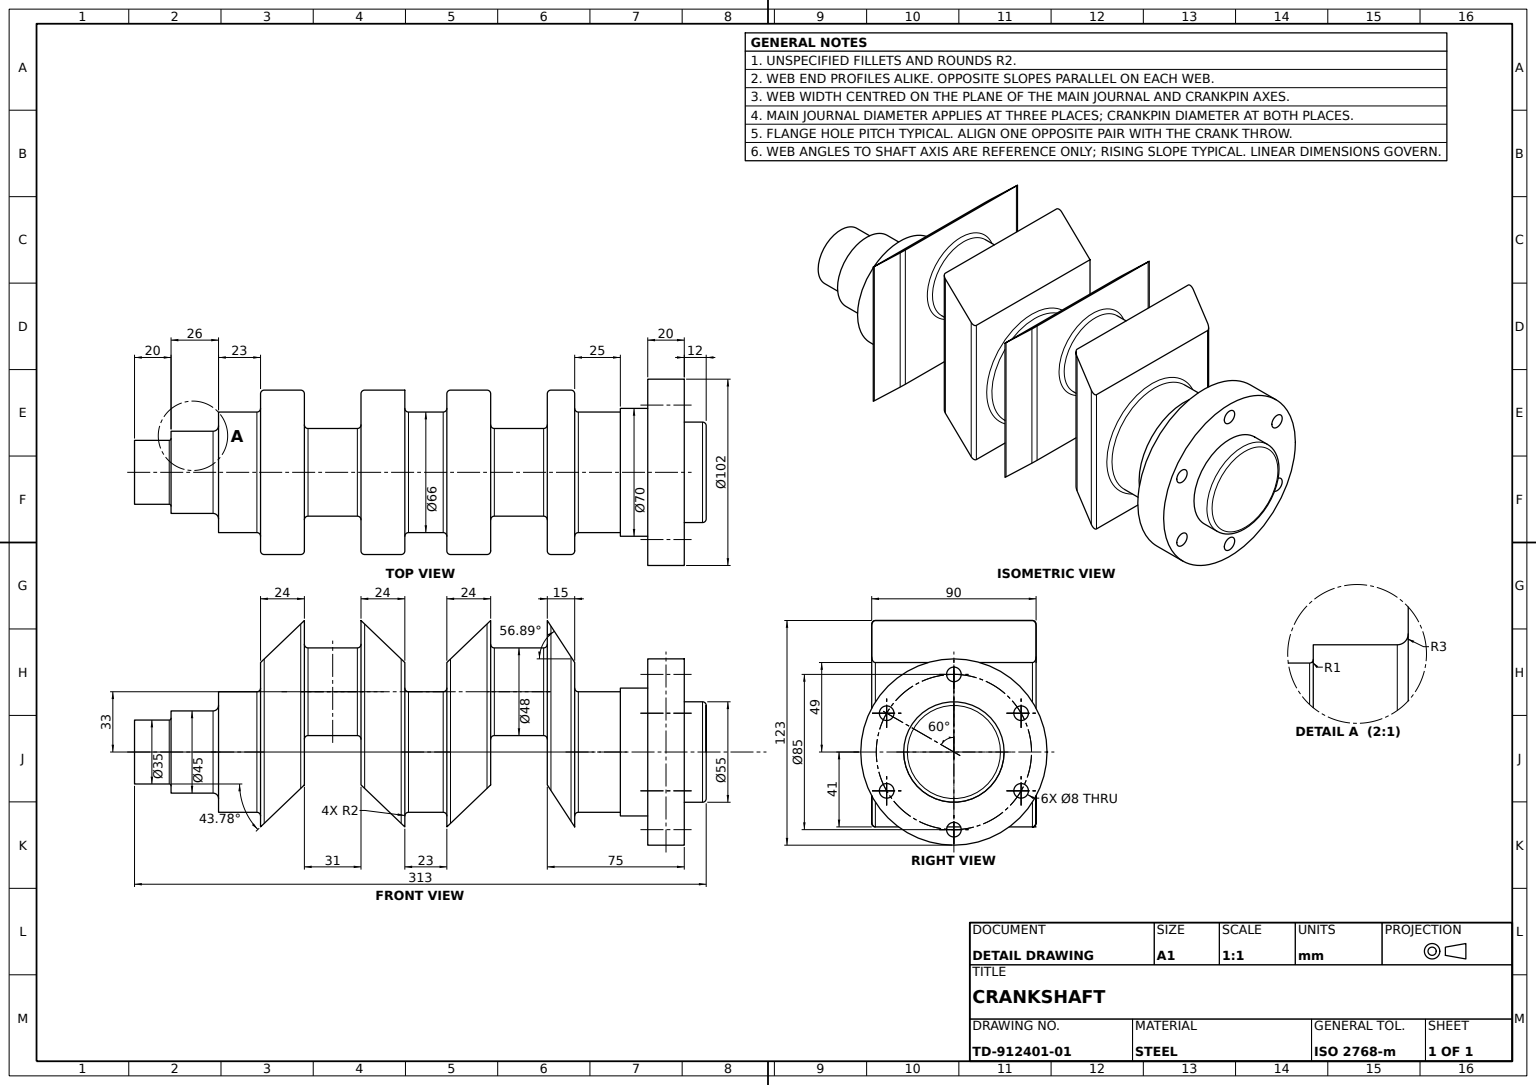
from build123d import *

# Parameters (mm, degrees)
FRONT_JOURNAL_35_SKETCH_R          = 17.5
FRONT_JOURNAL_35_DEPTH             = 20
SHAFT_STEP_45_SKETCH_R             = 22.5
SHAFT_STEP_45_DEPTH                = 26
FRONT_MAIN_JOURNAL_66_SKETCH_R     = 33
FRONT_MAIN_JOURNAL_66_DEPTH        = 23
CRANK_WEB_1_DEPTH                  = 45
CRANKPIN_1_48_SKETCH_R             = 24
CRANKPIN_1_48_DEPTH                = 31
CRANK_WEB_2_DEPTH                  = 45
CENTRE_MAIN_JOURNAL_66_SKETCH_R    = 33
CENTRE_MAIN_JOURNAL_66_DEPTH       = 23
CRANK_WEB_3_DEPTH                  = 45
CRANKPIN_2_SKETCH_R                = 24
CRANKPIN_2_DEPTH                   = 31
CRANK_WEB_4_DEPTH                  = 45
REAR_MAIN_JOURNAL_SKETCH_R         = 33
REAR_MAIN_JOURNAL_DEPTH            = 25
FLANGE_NECK_70_SKETCH_R            = 35
FLANGE_NECK_70_DEPTH               = 15
REAR_FLANGE_102_SKETCH_R           = 51
REAR_FLANGE_102_DEPTH              = 20
FLANGE_SPIGOT_55_SKETCH_R          = 27.5
FLANGE_SPIGOT_55_DEPTH             = 12
FLANGE_BOLT_HOLES_6X_8_PCD85_REACH = 315.665
FLANGE_BOLT_HOLES_SKETCH_R         = 4
FRONT_JOURNAL_FILLET_R1_R          = 1
SHAFT_STEP_FILLET_R3_R             = 3
JOURNAL_AND_CRANKPIN_FILLETS_R2_R  = 2
CRANK_WEB_1_EDGE_FILLET_R2_R       = 2
CRANK_WEBS_2_4_EDGE_FILLETS_R2_R   = 2


with BuildPart() as part:
    # Front Journal Ø35 Sketch → Front Journal Ø35 (new body)
    with BuildSketch(Plane.XY):
        Circle(FRONT_JOURNAL_35_SKETCH_R)
    extrude(amount=-FRONT_JOURNAL_35_DEPTH)

    # Shaft Step Ø45 Sketch → Shaft Step Ø45 (add)
    with BuildSketch(Plane(origin=(0, 0, -20), x_dir=(-1, 0, 0), z_dir=(0, 0, -1))):
        with Locations(Location((0, 0, 0), (0, 0, 180))):
            Circle(SHAFT_STEP_45_SKETCH_R)
    extrude(amount=SHAFT_STEP_45_DEPTH)

    # Front Main Journal Ø66 Sketch → Front Main Journal Ø66 (add)
    with BuildSketch(Plane(origin=(0, 0, -46), x_dir=(-1, 0, 0), z_dir=(0, 0, -1))):
        Circle(FRONT_MAIN_JOURNAL_66_SKETCH_R)
    extrude(amount=FRONT_MAIN_JOURNAL_66_DEPTH)

    # Crank Web 1 Profile → Crank Web 1 (add, symmetric)
    with BuildSketch(Plane(origin=(0, 0, 0), x_dir=(0, 0, -1), z_dir=(1, 0, 0))):
        Polygon((69, 0), (69, 49), (93, 72), (93, -18), (69, -41), align=None)
    extrude(amount=CRANK_WEB_1_DEPTH, both=True)

    # Crankpin 1 Ø48 Sketch → Crankpin 1 Ø48 (add)
    with BuildSketch(Plane(origin=(0, 0, -93), x_dir=(-1, 0, 0), z_dir=(0, 0, -1))):
        with Locations(Location((0, 33, 0), (0, 0, 90))):
            Circle(CRANKPIN_1_48_SKETCH_R)
    extrude(amount=CRANKPIN_1_48_DEPTH)

    # Crank Web 2 Profile → Crank Web 2 (add, symmetric)
    with BuildSketch(Plane(origin=(0, 0, 0), x_dir=(0, 0, -1), z_dir=(1, 0, 0))):
        Polygon((124, 72), (124, -18), (148, -41), (148, 49), align=None)
    extrude(amount=CRANK_WEB_2_DEPTH, both=True)

    # Centre Main Journal Ø66 Sketch → Centre Main Journal Ø66 (add)
    with BuildSketch(Plane(origin=(0, 0, -148), x_dir=(-1, 0, 0), z_dir=(0, 0, -1))):
        Circle(CENTRE_MAIN_JOURNAL_66_SKETCH_R)
    extrude(amount=CENTRE_MAIN_JOURNAL_66_DEPTH)

    # Crank Web 3 Profile → Crank Web 3 (add, symmetric)
    with BuildSketch(Plane(origin=(0, 0, 0), x_dir=(0, 0, -1), z_dir=(1, 0, 0))):
        Polygon((171, 0), (171, 49), (195, 72), (195, -18), (171, -41), align=None)
    extrude(amount=CRANK_WEB_3_DEPTH, both=True)

    # Crankpin 2 Sketch → Crankpin 2 (add)
    with BuildSketch(Plane(origin=(0, 0, -195), x_dir=(-1, 0, 0), z_dir=(0, 0, -1))):
        with Locations(Location((0, 33, 0), (0, 0, 90))):
            Circle(CRANKPIN_2_SKETCH_R)
    extrude(amount=CRANKPIN_2_DEPTH)

    # Crank Web 4 Profile → Crank Web 4 (add, symmetric)
    with BuildSketch(Plane(origin=(0, 0, 0), x_dir=(0, 0, -1), z_dir=(1, 0, 0))):
        Polygon((226, 57), (226, 72), (241, 49), (241, -41), (226, -18), align=None)
    extrude(amount=CRANK_WEB_4_DEPTH, both=True)

    # Rear Main Journal Sketch → Rear Main Journal (add)
    with BuildSketch(Plane(origin=(0, 0, -241), x_dir=(-1, 0, 0), z_dir=(0, 0, -1))):
        Circle(REAR_MAIN_JOURNAL_SKETCH_R)
    extrude(amount=REAR_MAIN_JOURNAL_DEPTH)

    # Flange Neck Ø70 Sketch → Flange Neck Ø70 (add)
    with BuildSketch(Plane(origin=(0, 0, -266), x_dir=(-1, 0, 0), z_dir=(0, 0, -1))):
        Circle(FLANGE_NECK_70_SKETCH_R)
    extrude(amount=FLANGE_NECK_70_DEPTH)

    # Rear Flange Ø102 Sketch → Rear Flange Ø102 (add)
    with BuildSketch(Plane(origin=(0, 0, -281), x_dir=(-1, 0, 0), z_dir=(0, 0, -1))):
        Circle(REAR_FLANGE_102_SKETCH_R)
    extrude(amount=REAR_FLANGE_102_DEPTH)

    # Flange Spigot Ø55 Sketch → Flange Spigot Ø55 (add)
    with BuildSketch(Plane(origin=(0, 0, -301), x_dir=(-1, 0, 0), z_dir=(0, 0, -1))):
        Circle(FLANGE_SPIGOT_55_SKETCH_R)
    extrude(amount=FLANGE_SPIGOT_55_DEPTH)

    # Flange Bolt Holes Sketch → Flange Bolt Holes 6xØ8 PCD85 (cut, up to next)
    with BuildSketch(Plane(origin=(0, 0, -301), x_dir=(-1, 0, 0), z_dir=(0, 0, -1)), mode=Mode.PRIVATE) as flange_bolt_holes_6x_8_pcd85_sk1:
        with Locations((0, 42.5)):
            Circle(FLANGE_BOLT_HOLES_SKETCH_R)
    flange_bolt_holes_6x_8_pcd85_tool1 = extrude(flange_bolt_holes_6x_8_pcd85_sk1.sketch, amount=-FLANGE_BOLT_HOLES_6X_8_PCD85_REACH, mode=Mode.PRIVATE) & part.part
    # Flange Bolt Holes Sketch → Flange Bolt Holes 6xØ8 PCD85 (cut, up to next)
    with BuildSketch(Plane(origin=(0, 0, -301), x_dir=(-1, 0, 0), z_dir=(0, 0, -1)), mode=Mode.PRIVATE) as flange_bolt_holes_6x_8_pcd85_sk2:
        with Locations((36.806079661, 21.25)):
            Circle(FLANGE_BOLT_HOLES_SKETCH_R)
    flange_bolt_holes_6x_8_pcd85_tool2 = extrude(flange_bolt_holes_6x_8_pcd85_sk2.sketch, amount=-FLANGE_BOLT_HOLES_6X_8_PCD85_REACH, mode=Mode.PRIVATE) & part.part
    # Flange Bolt Holes Sketch → Flange Bolt Holes 6xØ8 PCD85 (cut, up to next)
    with BuildSketch(Plane(origin=(0, 0, -301), x_dir=(-1, 0, 0), z_dir=(0, 0, -1)), mode=Mode.PRIVATE) as flange_bolt_holes_6x_8_pcd85_sk3:
        with Locations((36.806079661, -21.25)):
            Circle(FLANGE_BOLT_HOLES_SKETCH_R)
    flange_bolt_holes_6x_8_pcd85_tool3 = extrude(flange_bolt_holes_6x_8_pcd85_sk3.sketch, amount=-FLANGE_BOLT_HOLES_6X_8_PCD85_REACH, mode=Mode.PRIVATE) & part.part
    # Flange Bolt Holes Sketch → Flange Bolt Holes 6xØ8 PCD85 (cut, up to next)
    with BuildSketch(Plane(origin=(0, 0, -301), x_dir=(-1, 0, 0), z_dir=(0, 0, -1)), mode=Mode.PRIVATE) as flange_bolt_holes_6x_8_pcd85_sk4:
        with Locations((0, -42.5)):
            Circle(FLANGE_BOLT_HOLES_SKETCH_R)
    flange_bolt_holes_6x_8_pcd85_tool4 = extrude(flange_bolt_holes_6x_8_pcd85_sk4.sketch, amount=-FLANGE_BOLT_HOLES_6X_8_PCD85_REACH, mode=Mode.PRIVATE) & part.part
    # Flange Bolt Holes Sketch → Flange Bolt Holes 6xØ8 PCD85 (cut, up to next)
    with BuildSketch(Plane(origin=(0, 0, -301), x_dir=(-1, 0, 0), z_dir=(0, 0, -1)), mode=Mode.PRIVATE) as flange_bolt_holes_6x_8_pcd85_sk5:
        with Locations((-36.806079661, -21.25)):
            Circle(FLANGE_BOLT_HOLES_SKETCH_R)
    flange_bolt_holes_6x_8_pcd85_tool5 = extrude(flange_bolt_holes_6x_8_pcd85_sk5.sketch, amount=-FLANGE_BOLT_HOLES_6X_8_PCD85_REACH, mode=Mode.PRIVATE) & part.part
    # Flange Bolt Holes Sketch → Flange Bolt Holes 6xØ8 PCD85 (cut, up to next)
    with BuildSketch(Plane(origin=(0, 0, -301), x_dir=(-1, 0, 0), z_dir=(0, 0, -1)), mode=Mode.PRIVATE) as flange_bolt_holes_6x_8_pcd85_sk6:
        with Locations((-36.806079661, 21.25)):
            Circle(FLANGE_BOLT_HOLES_SKETCH_R)
    flange_bolt_holes_6x_8_pcd85_tool6 = extrude(flange_bolt_holes_6x_8_pcd85_sk6.sketch, amount=-FLANGE_BOLT_HOLES_6X_8_PCD85_REACH, mode=Mode.PRIVATE) & part.part
    add(flange_bolt_holes_6x_8_pcd85_tool1.solids().sort_by_distance((0, 42.5, -301))[0], mode=Mode.SUBTRACT)
    add(flange_bolt_holes_6x_8_pcd85_tool2.solids().sort_by_distance((-36.80608, 21.25, -301))[0], mode=Mode.SUBTRACT)
    add(flange_bolt_holes_6x_8_pcd85_tool3.solids().sort_by_distance((-36.80608, -21.25, -301))[0], mode=Mode.SUBTRACT)
    add(flange_bolt_holes_6x_8_pcd85_tool4.solids().sort_by_distance((0, -42.5, -301))[0], mode=Mode.SUBTRACT)
    add(flange_bolt_holes_6x_8_pcd85_tool5.solids().sort_by_distance((36.80608, -21.25, -301))[0], mode=Mode.SUBTRACT)
    add(flange_bolt_holes_6x_8_pcd85_tool6.solids().sort_by_distance((36.80608, 21.25, -301))[0], mode=Mode.SUBTRACT)

    # Front Journal Fillet R1
    front_journal_fillet_r1_edges = [part.edges().sort_by_distance(p)[0] for p in [
        (-17.5, 0, -20),
    ]]
    fillet(front_journal_fillet_r1_edges, radius=FRONT_JOURNAL_FILLET_R1_R)

    # Shaft Step Fillet R3
    shaft_step_fillet_r3_edges = [part.edges().sort_by_distance(p)[0] for p in [
        (-22.5, 0, -46),
    ]]
    fillet(shaft_step_fillet_r3_edges, radius=SHAFT_STEP_FILLET_R3_R)

    # Journal and Crankpin Fillets R2
    journal_and_crankpin_fillets_r2_edges = [part.edges().sort_by_distance(p)[0] for p in [
        (33, 0, -69),
        (0, 9, -93),
        (0, 9, -124),
        (33, 0, -148),
        (33, 0, -171),
        (0, 9, -195),
        (0, 9, -226),
        (33, 0, -241),
        (27.5, 0, -313),
    ]]
    fillet(journal_and_crankpin_fillets_r2_edges, radius=JOURNAL_AND_CRANKPIN_FILLETS_R2_R)

    # Crank Web 1 Edge Fillet R2
    crank_web_1_edge_fillet_r2_edges = [part.edges().sort_by_distance(p)[0] for p in [
        (-45, 27, -93),
        (-45, 4, -69),
        (45, 4, -69),
        (45, 27, -93),
    ]]
    fillet(crank_web_1_edge_fillet_r2_edges, radius=CRANK_WEB_1_EDGE_FILLET_R2_R)

    # Crank Webs 2-4 Edge Fillets R2
    crank_webs_2_4_edge_fillets_r2_edges = [part.edges().sort_by_distance(p)[0] for p in [
        (-45, 27, -124),
        (45, 27, -124),
        (45, 4, -148),
        (-45, 27, -195),
        (-45, 4, -171),
        (45, 4, -171),
        (45, 27, -195),
        (-45, 4, -241),
        (-45, 27, -226),
        (45, 27, -226),
        (45, 4, -241),
    ]]
    fillet(crank_webs_2_4_edge_fillets_r2_edges, radius=CRANK_WEBS_2_4_EDGE_FILLETS_R2_R)


solid = part.part
